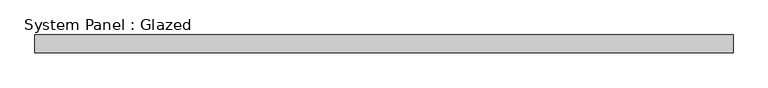
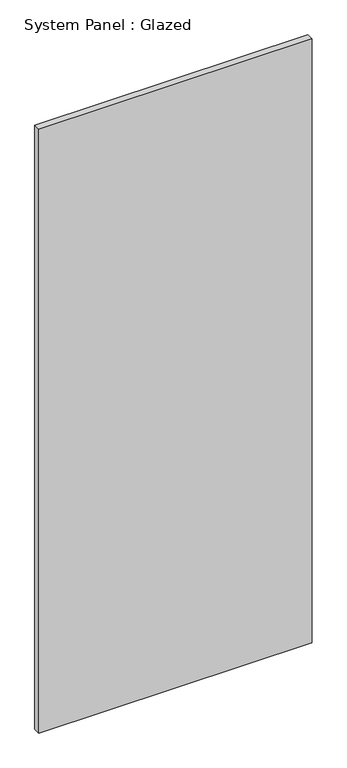
"""IFC4 building model written with IfcOpenShell, lengths in millimetres: plate geometry, System Panel : Glazed."""

from ifc_helpers import new_model, si_unit, origin, origin_with_axes, place, context, project, spatial, polyline, outline, extrude, source, transform, mapped, element, save


def system_panel_glazed_ee97838a(model_context):
    return source(origin(), model_context, "Body", "SweptSolid", [
        extrude(outline(polyline([(501.6499999, 19.05), (-501.6499999, 19.05), (-501.6499999, 44.45), (501.6499999, 44.45), (501.6499999, 19.05)])), origin_with_axes(), (0.0, 0.0, 1.0), 2343.15),
    ])


if __name__ == "__main__":
    model = new_model("IFC4")
    model_context = context("Model", 3, world=origin())
    ifc_project = project(units=[si_unit("LENGTHUNIT", "METRE", prefix="MILLI")], contexts=[model_context])
    site = spatial("IfcSite", under=ifc_project)
    building = spatial("IfcBuilding", under=site)
    placement = place(None, origin())
    system_panel_glazed_shape = system_panel_glazed_ee97838a(model_context)
    element("IfcPlate", 1, ObjectType="System Panel : Glazed", at=placement, inside=building, context=model_context, shape_type="MappedRepresentation", body=[
        mapped(system_panel_glazed_shape, transform((0.0, 0.0, 0.0), x_axis=(1.0, 0.0, 0.0), y_axis=(0.0, 1.0, 0.0), z_axis=(0.0, 0.0, 1.0))),
    ])
    save(model, "model.ifc")

# Revit data of these elements
# Type "System Panel : Glazed"
#   Construction Type Id = "GSP4R"
#   Analytic Construction = "1/8 in Pilkington single glazing"
#   Visual Light Transmittance = 0.9
#   Solar Heat Gain Coefficient = 0.86
#   Heat Transfer Coefficient (U) = 1.18115 BTU/(h·ft²·°F)
#   Define Thermal Properties by = 1
# Element 1 (IfcPlate, "System Panel : Glazed")
#   Materials on its faces: "Glass"
# Materials
#   "Glass": class "Glass", colour RGB 0 128 192, transparency 0.75, Description = "Soda Lime Glass", Cost = 0
